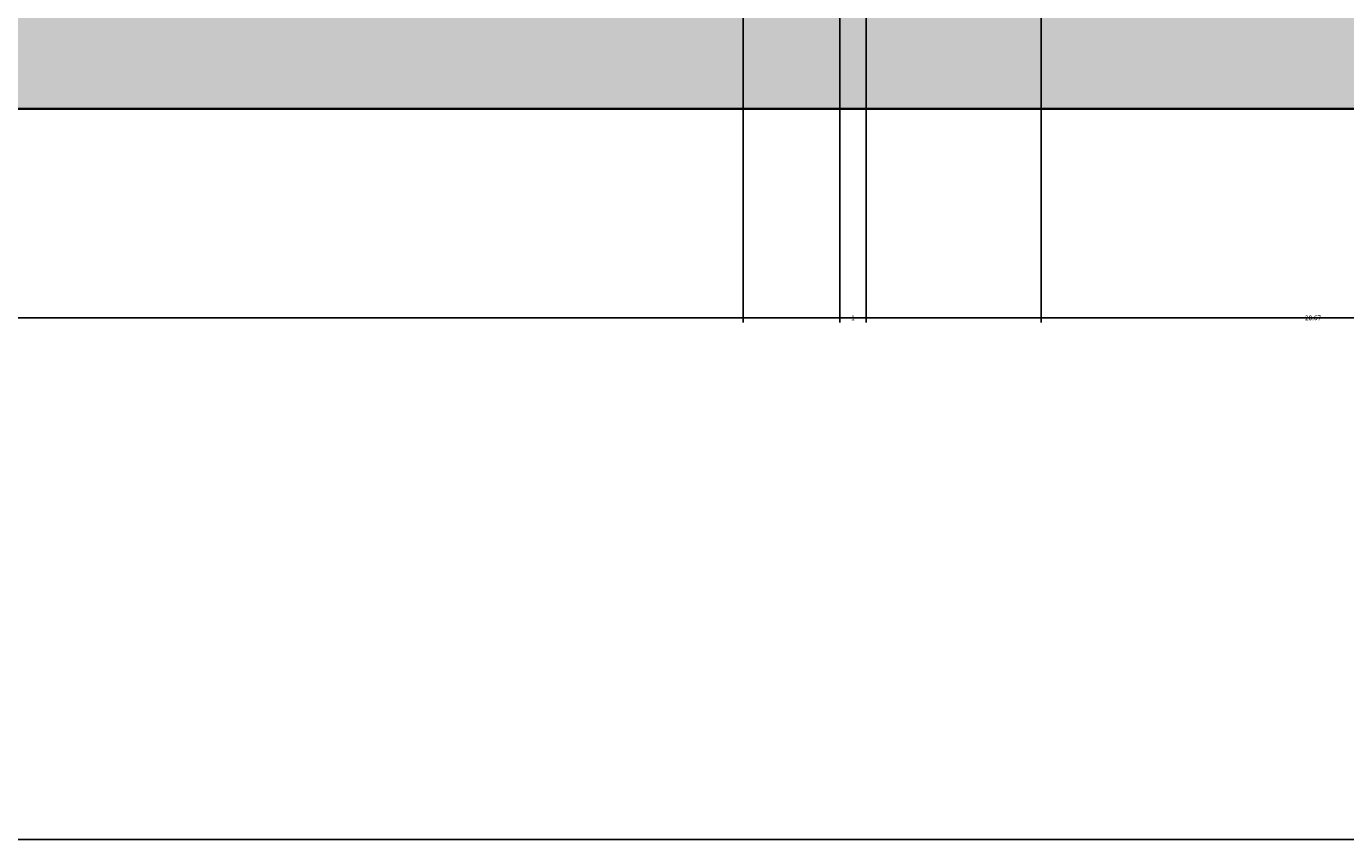
# Model space of a CAD drawing. Units: inches. Extents: x 4508 to 4723, y 847 to 1020.
# Tile 18 of 32: x 4631 to 4681, y 847 to 878. Entities that reach past the tile are written whole.
import ezdxf

# ---------------------------------------------------------------- set-up
doc = ezdxf.new("R2010")
doc.units = ezdxf.units.IN
for name, color, linetype, lineweight in [('A-ANNO-DIMS', 2, 'Continuous', 18), ('A-ANNO-TTLB', 7, 'Continuous', 25), ('A-WALL', 7, 'Continuous', 35), ('A-WALL-PATT', 254, 'Continuous', 13)]:
    doc.layers.add(name, color=color, linetype=linetype, lineweight=lineweight)
doc.styles.get("Standard").update_dxf_attribs({"font": 'arial.ttf'})
doc.dimstyles.get("Standard").update_dxf_attribs({"dimtxt": 0.18, "dimasz": 0.18, "dimexe": 0.18, "dimexo": 0.0625, "dimgap": 0.09, "dimtad": 0, "dimtih": 1, "dimtoh": 1, "dimdec": 4, "dimzin": 0, "dimdsep": 46, "dimtxsty": 'Standard', "dimcen": 0.09, "dimadec": 0, "dimazin": 0, "dimtfac": 1, "dimtdec": 4, "dimtofl": 0, "dimtmove": 0, "dimatfit": 3, "dimfxl": 1, "dimtolj": 1, "dimtzin": 0, "dimarcsym": 0})

# ---------------------------------------------------------------- blocks, each defined once
blk = doc.blocks.new('*D2')
at = {"layer": 'A-ANNO-DIMS', "color": 0, "lineweight": -2, "transparency": 16777216}
for p, q in [((4540.994, 874.684), (4540.994, 866.617)), ((4693.994, 874.684), (4693.994, 866.617)), ((4541.174, 866.797), (4617.213, 866.797)), ((4693.814, 866.797), (4617.774, 866.797))]:
    blk.add_line(p, q, dxfattribs=at)
at = {"layer": 'A-ANNO-DIMS', "color": 0, "lineweight": 9, "transparency": 16777216}
for points in [[(4541.174, 866.827), (4541.174, 866.767), (4540.994, 866.797)], [(4693.814, 866.827), (4693.814, 866.767), (4693.994, 866.797)]]:
    blk.add_solid(points, dxfattribs=at)
at = {"layer": 'Defpoints', "color": 0, "lineweight": 9, "transparency": 16777216}
for p in [(4540.994, 874.747), (4693.994, 874.747), (4693.994, 866.797)]:
    blk.add_point(p, dxfattribs=at)
at = {"layer": 'A-ANNO-DIMS', "color": 0, "transparency": 16777216, "insert": (4617.494, 866.797), "char_height": 0.18, "attachment_point": 5}
blk.add_mtext('\\A1;153', dxfattribs=at)
blk = doc.blocks.new('*D13')
at = {"layer": 'A-ANNO-DIMS', "color": 0, "lineweight": -2, "transparency": 16777216}
for p, q in [((4669.325, 973.916), (4669.325, 866.617)), ((4689.994, 874.684), (4689.994, 866.617)), ((4669.505, 866.797), (4679.264, 866.797)), ((4689.814, 866.797), (4680.054, 866.797))]:
    blk.add_line(p, q, dxfattribs=at)
at = {"layer": 'A-ANNO-DIMS', "color": 0, "lineweight": 9, "transparency": 16777216}
for points in [[(4669.505, 866.827), (4669.505, 866.767), (4669.325, 866.797)], [(4689.814, 866.827), (4689.814, 866.767), (4689.994, 866.797)]]:
    blk.add_solid(points, dxfattribs=at)
at = {"layer": 'Defpoints', "color": 0, "lineweight": 9, "transparency": 16777216}
for p in [(4669.325, 973.978), (4689.994, 874.747), (4689.994, 866.797)]:
    blk.add_point(p, dxfattribs=at)
at = {"layer": 'A-ANNO-DIMS', "color": 0, "transparency": 16777216, "insert": (4679.659, 866.797), "char_height": 0.18, "attachment_point": 5}
blk.add_mtext('\\A1;20.67', dxfattribs=at)
blk = doc.blocks.new('*D15')
at = {"layer": 'A-ANNO-DIMS', "color": 0, "lineweight": -2, "transparency": 16777216}
for p, q in [((4661.671, 918.138), (4661.671, 866.617)), ((4662.671, 918.138), (4662.671, 866.617)), ((4661.851, 866.797), (4662.047, 866.797)), ((4662.491, 866.797), (4662.294, 866.797))]:
    blk.add_line(p, q, dxfattribs=at)
at = {"layer": 'A-ANNO-DIMS', "color": 0, "lineweight": 9, "transparency": 16777216}
for points in [[(4661.851, 866.827), (4661.851, 866.767), (4661.671, 866.797)], [(4662.491, 866.827), (4662.491, 866.767), (4662.671, 866.797)]]:
    blk.add_solid(points, dxfattribs=at)
at = {"layer": 'Defpoints', "color": 0, "lineweight": 9, "transparency": 16777216}
for p in [(4661.671, 918.2), (4662.671, 918.2), (4662.671, 866.797)]:
    blk.add_point(p, dxfattribs=at)
at = {"layer": 'A-ANNO-DIMS', "color": 0, "transparency": 16777216, "insert": (4662.171, 866.797), "char_height": 0.18, "attachment_point": 5}
blk.add_mtext('\\A1;1', dxfattribs=at)
blk = doc.blocks.new('*D24')
at = {"layer": 'A-ANNO-DIMS', "color": 0, "lineweight": -2, "transparency": 16777216}
for p, q in [((4549.994, 886.684), (4549.994, 866.617)), ((4657.994, 886.684), (4657.994, 866.617)), ((4550.174, 866.797), (4603.713, 866.797)), ((4657.814, 866.797), (4604.274, 866.797))]:
    blk.add_line(p, q, dxfattribs=at)
at = {"layer": 'A-ANNO-DIMS', "color": 0, "lineweight": 9, "transparency": 16777216}
for points in [[(4550.174, 866.827), (4550.174, 866.767), (4549.994, 866.797)], [(4657.814, 866.827), (4657.814, 866.767), (4657.994, 866.797)]]:
    blk.add_solid(points, dxfattribs=at)
at = {"layer": 'Defpoints', "color": 0, "lineweight": 9, "transparency": 16777216}
for p in [(4549.994, 886.747), (4657.994, 886.747), (4657.994, 866.797)]:
    blk.add_point(p, dxfattribs=at)
at = {"layer": 'A-ANNO-DIMS', "color": 0, "transparency": 16777216, "insert": (4603.994, 866.797), "char_height": 0.18, "attachment_point": 5}
blk.add_mtext('\\A1;108', dxfattribs=at)

msp = doc.modelspace()

# ---------------------------------------------------------------- hatches: boundary and pattern name
at = {"layer": 'A-WALL-PATT', "transparency": 33554556}
h = msp.add_hatch(color=256, dxfattribs=at)
h.dxf.hatch_style = 1
h.paths.add_polyline_path([(4689.9938, 878.7469), (4549.9938, 878.7469), (4549.9938, 874.7469), (4689.9938, 874.7469)])

# ---------------------------------------------------------------- linework, layer by layer
at = {"layer": 'A-ANNO-TTLB'}
msp.add_lwpolyline([(4508.3867, 1019.9118), (4722.9774, 1019.9118), (4722.9774, 846.9535), (4508.3867, 846.9535)], close=True, dxfattribs=at)
at = {"layer": 'A-WALL'}
msp.add_line((4693.9938, 874.7469), (4549.9938, 874.7469), dxfattribs=at)

# ---------------------------------------------------------------- dimensions: what is measured, and where the dimension line sits
at = {"layer": 'A-ANNO-DIMS'}
for base, p1, p2, override, picture, middle in [((4689.9938, 866.7969), (4669.3246, 973.9783), (4689.9938, 874.7469), {"dimdec": 2, "dimlfac": 1, "dimrnd": 0, "dimzin": 0, "dimdsep": 46, "dimlunit": 2}, '*D13', (4679.6592, 866.7969)), ((4662.6706, 866.7969), (4661.6706, 918.2003), (4662.6706, 918.2003), {"dimdec": 0, "dimlfac": 1, "dimrnd": 0, "dimzin": 0, "dimdsep": 46, "dimlunit": 2}, '*D15', (4662.1706, 866.7969)), ((4657.9938, 866.7969), (4549.9938, 886.7469), (4657.9938, 886.7469), {"dimdec": 0, "dimlfac": 1, "dimrnd": 0, "dimzin": 0, "dimdsep": 46, "dimlunit": 2}, '*D24', (4603.9938, 866.7969)), ((4693.9938, 866.7969), (4540.9938, 874.7469), (4693.9938, 874.7469), {"dimdec": 0, "dimlfac": 1, "dimrnd": 0, "dimzin": 0, "dimdsep": 46, "dimlunit": 2}, '*D2', (4617.4938, 866.7969))]:
    dim = msp.add_linear_dim(base=base, p1=p1, p2=p2, dimstyle='Standard', override=override, dxfattribs=at)
    dim.commit()
    dim.dimension.update_dxf_attribs({"geometry": picture, "text_midpoint": middle})

doc.saveas('drawing.dxf')
